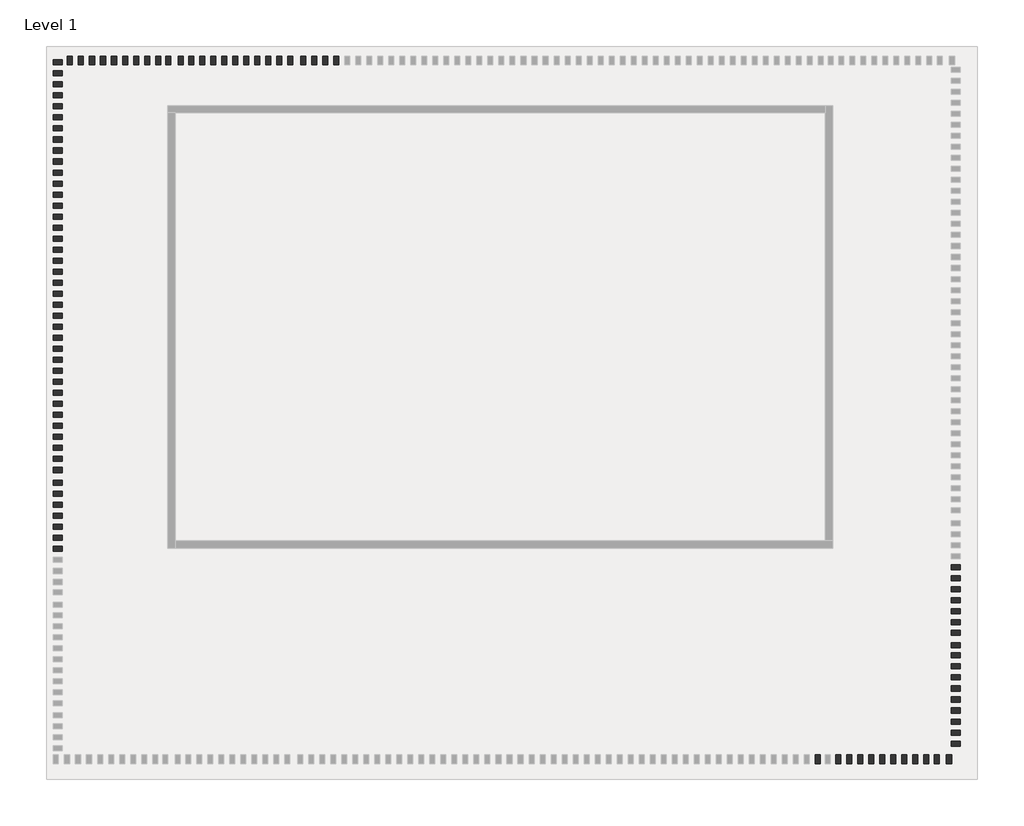
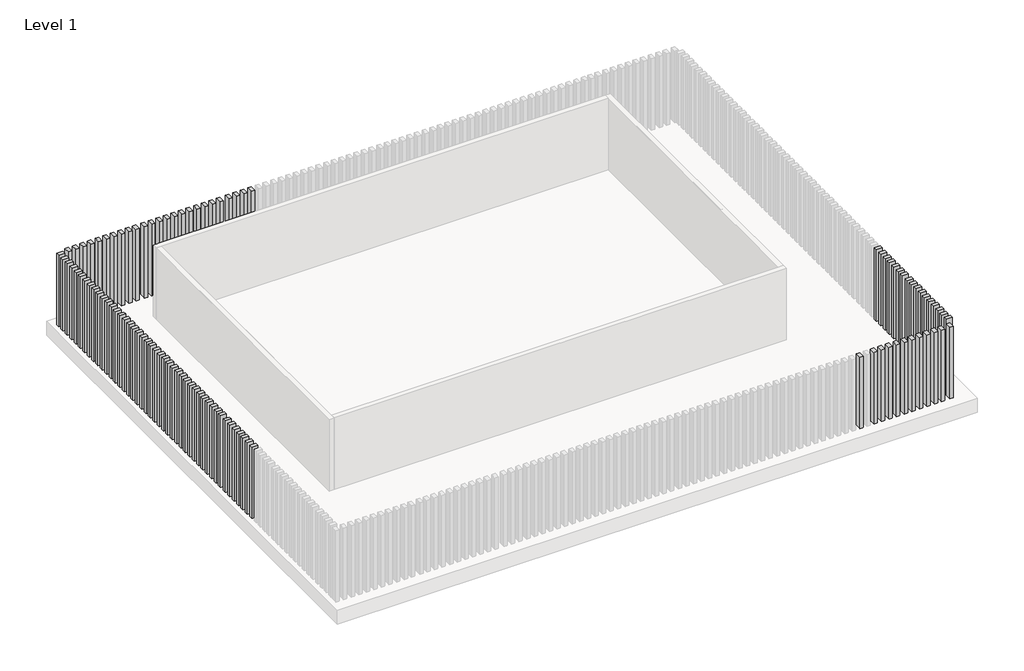
# One storey, part 2 of 3: 99 columns.
"""IFC4 building model written with IfcOpenShell, lengths in millimetres."""

from ifc_helpers import new_model, si_unit, origin, place, context, project, spatial, transform, mapped, element, save
from components import wood_timber_column_6_x_10_8585acab

model = new_model("IFC4")

# Units and contexts
model_context = context("Model", 3, world=origin())
ifc_project = project(units=[si_unit("LENGTHUNIT", "METRE", prefix="MILLI")], contexts=[model_context])

# Site, building, storey
site = spatial("IfcSite", under=ifc_project)
building = spatial("IfcBuilding", under=site)
storey = spatial("IfcBuildingStorey", under=building, Name="Level 1", Elevation=0.0)

# Columns
placement = place(None, origin())
wood_timber_column_6_x_10_shape = wood_timber_column_6_x_10_8585acab(model_context)
element("IfcColumn", 1, ObjectType="Wood Timber Column : 6 x 10", at=placement, inside=storey, context=model_context, shape_type="MappedRepresentation", body=[
    mapped(wood_timber_column_6_x_10_shape, transform((2270.6466756, -5612.3567338, 0.0), x_axis=(1.0, 0.0, 0.0), y_axis=(0.0, 1.0, 0.0), z_axis=(0.0, 0.0, 1.0))),
])
element("IfcColumn", 2, ObjectType="Wood Timber Column : 6 x 10", at=placement, inside=storey, context=model_context, shape_type="MappedRepresentation", body=[
    mapped(wood_timber_column_6_x_10_shape, transform((-18761.0148275, 13665.8652966, 0.0), x_axis=(0.0, 1.0, 0.0), y_axis=(-1.0000000000000002, 0.0, 0.0), z_axis=(0.0, 0.0, 1.0000000000000002))),
])
element("IfcColumn", 3, ObjectType="Wood Timber Column : 6 x 10", at=placement, inside=storey, context=model_context, shape_type="MappedRepresentation", body=[
    mapped(wood_timber_column_6_x_10_shape, transform((-18761.0148275, 13361.0652966, 0.0), x_axis=(0.0, 1.0, 0.0), y_axis=(-1.0000000000000002, 0.0, 0.0), z_axis=(0.0, 0.0, 1.0000000000000002))),
])
element("IfcColumn", 4, ObjectType="Wood Timber Column : 6 x 10", at=placement, inside=storey, context=model_context, shape_type="MappedRepresentation", body=[
    mapped(wood_timber_column_6_x_10_shape, transform((-18761.0148275, 13056.2652966, 0.0), x_axis=(0.0, 1.0, 0.0), y_axis=(-1.0000000000000002, 0.0, 0.0), z_axis=(0.0, 0.0, 1.0000000000000002))),
])
element("IfcColumn", 5, ObjectType="Wood Timber Column : 6 x 10", at=placement, inside=storey, context=model_context, shape_type="MappedRepresentation", body=[
    mapped(wood_timber_column_6_x_10_shape, transform((-18761.0148275, 12751.4652966, 0.0), x_axis=(0.0, 1.0, 0.0), y_axis=(-1.0000000000000002, 0.0, 0.0), z_axis=(0.0, 0.0, 1.0000000000000002))),
])
element("IfcColumn", 6, ObjectType="Wood Timber Column : 6 x 10", at=placement, inside=storey, context=model_context, shape_type="MappedRepresentation", body=[
    mapped(wood_timber_column_6_x_10_shape, transform((-18761.0148275, 12446.6652966, 0.0), x_axis=(0.0, 1.0, 0.0), y_axis=(-1.0000000000000002, 0.0, 0.0), z_axis=(0.0, 0.0, 1.0000000000000002))),
])
element("IfcColumn", 7, ObjectType="Wood Timber Column : 6 x 10", at=placement, inside=storey, context=model_context, shape_type="MappedRepresentation", body=[
    mapped(wood_timber_column_6_x_10_shape, transform((-18761.0148275, 12141.8652966, 0.0), x_axis=(0.0, 1.0, 0.0), y_axis=(-1.0000000000000002, 0.0, 0.0), z_axis=(0.0, 0.0, 1.0000000000000002))),
])
element("IfcColumn", 8, ObjectType="Wood Timber Column : 6 x 10", at=placement, inside=storey, context=model_context, shape_type="MappedRepresentation", body=[
    mapped(wood_timber_column_6_x_10_shape, transform((-18761.0148275, 11837.0652966, 0.0), x_axis=(0.0, 1.0, 0.0), y_axis=(-1.0000000000000002, 0.0, 0.0), z_axis=(0.0, 0.0, 1.0000000000000002))),
])
element("IfcColumn", 9, ObjectType="Wood Timber Column : 6 x 10", at=placement, inside=storey, context=model_context, shape_type="MappedRepresentation", body=[
    mapped(wood_timber_column_6_x_10_shape, transform((-18761.0148275, 11532.2652966, 0.0), x_axis=(0.0, 1.0, 0.0), y_axis=(-1.0000000000000002, 0.0, 0.0), z_axis=(0.0, 0.0, 1.0000000000000002))),
])
element("IfcColumn", 10, ObjectType="Wood Timber Column : 6 x 10", at=placement, inside=storey, context=model_context, shape_type="MappedRepresentation", body=[
    mapped(wood_timber_column_6_x_10_shape, transform((-18761.0148275, 11227.4652966, 0.0), x_axis=(0.0, 1.0, 0.0), y_axis=(-1.0000000000000002, 0.0, 0.0), z_axis=(0.0, 0.0, 1.0000000000000002))),
])
element("IfcColumn", 11, ObjectType="Wood Timber Column : 6 x 10", at=placement, inside=storey, context=model_context, shape_type="MappedRepresentation", body=[
    mapped(wood_timber_column_6_x_10_shape, transform((-18761.0148275, 10922.6652966, 0.0), x_axis=(0.0, 1.0, 0.0), y_axis=(-1.0000000000000002, 0.0, 0.0), z_axis=(0.0, 0.0, 1.0000000000000002))),
])
element("IfcColumn", 12, ObjectType="Wood Timber Column : 6 x 10", at=placement, inside=storey, context=model_context, shape_type="MappedRepresentation", body=[
    mapped(wood_timber_column_6_x_10_shape, transform((-18761.0148275, 10617.8652966, 0.0), x_axis=(0.0, 1.0, 0.0), y_axis=(-1.0000000000000002, 0.0, 0.0), z_axis=(0.0, 0.0, 1.0000000000000002))),
])
element("IfcColumn", 13, ObjectType="Wood Timber Column : 6 x 10", at=placement, inside=storey, context=model_context, shape_type="MappedRepresentation", body=[
    mapped(wood_timber_column_6_x_10_shape, transform((-18761.0148275, 10313.0652966, 0.0), x_axis=(0.0, 1.0, 0.0), y_axis=(-1.0000000000000002, 0.0, 0.0), z_axis=(0.0, 0.0, 1.0000000000000002))),
])
element("IfcColumn", 14, ObjectType="Wood Timber Column : 6 x 10", at=placement, inside=storey, context=model_context, shape_type="MappedRepresentation", body=[
    mapped(wood_timber_column_6_x_10_shape, transform((-18761.0148275, 10008.2652966, 0.0), x_axis=(0.0, 1.0, 0.0), y_axis=(-1.0000000000000002, 0.0, 0.0), z_axis=(0.0, 0.0, 1.0000000000000002))),
])
element("IfcColumn", 15, ObjectType="Wood Timber Column : 6 x 10", at=placement, inside=storey, context=model_context, shape_type="MappedRepresentation", body=[
    mapped(wood_timber_column_6_x_10_shape, transform((-18761.0148275, 9703.4652966, 0.0), x_axis=(0.0, 1.0, 0.0), y_axis=(-1.0000000000000002, 0.0, 0.0), z_axis=(0.0, 0.0, 1.0000000000000002))),
])
element("IfcColumn", 16, ObjectType="Wood Timber Column : 6 x 10", at=placement, inside=storey, context=model_context, shape_type="MappedRepresentation", body=[
    mapped(wood_timber_column_6_x_10_shape, transform((-18761.0148275, 9398.6652966, 0.0), x_axis=(0.0, 1.0, 0.0), y_axis=(-1.0000000000000002, 0.0, 0.0), z_axis=(0.0, 0.0, 1.0000000000000002))),
])
element("IfcColumn", 17, ObjectType="Wood Timber Column : 6 x 10", at=placement, inside=storey, context=model_context, shape_type="MappedRepresentation", body=[
    mapped(wood_timber_column_6_x_10_shape, transform((-18761.0148275, 9093.8652966, 0.0), x_axis=(0.0, 1.0, 0.0), y_axis=(-1.0000000000000002, 0.0, 0.0), z_axis=(0.0, 0.0, 1.0000000000000002))),
])
element("IfcColumn", 18, ObjectType="Wood Timber Column : 6 x 10", at=placement, inside=storey, context=model_context, shape_type="MappedRepresentation", body=[
    mapped(wood_timber_column_6_x_10_shape, transform((-18761.0148275, 8789.0652966, 0.0), x_axis=(0.0, 1.0, 0.0), y_axis=(-1.0000000000000002, 0.0, 0.0), z_axis=(0.0, 0.0, 1.0000000000000002))),
])
element("IfcColumn", 19, ObjectType="Wood Timber Column : 6 x 10", at=placement, inside=storey, context=model_context, shape_type="MappedRepresentation", body=[
    mapped(wood_timber_column_6_x_10_shape, transform((-18761.0148275, 8484.2652966, 0.0), x_axis=(0.0, 1.0, 0.0), y_axis=(-1.0000000000000002, 0.0, 0.0), z_axis=(0.0, 0.0, 1.0000000000000002))),
])
element("IfcColumn", 20, ObjectType="Wood Timber Column : 6 x 10", at=placement, inside=storey, context=model_context, shape_type="MappedRepresentation", body=[
    mapped(wood_timber_column_6_x_10_shape, transform((-18761.0148275, 8179.4652966, 0.0), x_axis=(0.0, 1.0, 0.0), y_axis=(-1.0000000000000002, 0.0, 0.0), z_axis=(0.0, 0.0, 1.0000000000000002))),
])
element("IfcColumn", 21, ObjectType="Wood Timber Column : 6 x 10", at=placement, inside=storey, context=model_context, shape_type="MappedRepresentation", body=[
    mapped(wood_timber_column_6_x_10_shape, transform((-18761.0148275, 7874.6652966, 0.0), x_axis=(0.0, 1.0, 0.0), y_axis=(-1.0000000000000002, 0.0, 0.0), z_axis=(0.0, 0.0, 1.0000000000000002))),
])
element("IfcColumn", 22, ObjectType="Wood Timber Column : 6 x 10", at=placement, inside=storey, context=model_context, shape_type="MappedRepresentation", body=[
    mapped(wood_timber_column_6_x_10_shape, transform((-18761.0148275, 7569.8652966, 0.0), x_axis=(0.0, 1.0, 0.0), y_axis=(-1.0000000000000002, 0.0, 0.0), z_axis=(0.0, 0.0, 1.0000000000000002))),
])
element("IfcColumn", 23, ObjectType="Wood Timber Column : 6 x 10", at=placement, inside=storey, context=model_context, shape_type="MappedRepresentation", body=[
    mapped(wood_timber_column_6_x_10_shape, transform((-18761.0148275, 7265.0652966, 0.0), x_axis=(0.0, 1.0, 0.0), y_axis=(-1.0000000000000002, 0.0, 0.0), z_axis=(0.0, 0.0, 1.0000000000000002))),
])
element("IfcColumn", 24, ObjectType="Wood Timber Column : 6 x 10", at=placement, inside=storey, context=model_context, shape_type="MappedRepresentation", body=[
    mapped(wood_timber_column_6_x_10_shape, transform((-18761.0148275, 6960.2652966, 0.0), x_axis=(0.0, 1.0, 0.0), y_axis=(-1.0000000000000002, 0.0, 0.0), z_axis=(0.0, 0.0, 1.0000000000000002))),
])
element("IfcColumn", 25, ObjectType="Wood Timber Column : 6 x 10", at=placement, inside=storey, context=model_context, shape_type="MappedRepresentation", body=[
    mapped(wood_timber_column_6_x_10_shape, transform((-18761.0148275, 6655.4652966, 0.0), x_axis=(0.0, 1.0, 0.0), y_axis=(-1.0000000000000002, 0.0, 0.0), z_axis=(0.0, 0.0, 1.0000000000000002))),
])
element("IfcColumn", 26, ObjectType="Wood Timber Column : 6 x 10", at=placement, inside=storey, context=model_context, shape_type="MappedRepresentation", body=[
    mapped(wood_timber_column_6_x_10_shape, transform((-18761.0148275, 6350.6652966, 0.0), x_axis=(0.0, 1.0, 0.0), y_axis=(-1.0000000000000002, 0.0, 0.0), z_axis=(0.0, 0.0, 1.0000000000000002))),
])
element("IfcColumn", 27, ObjectType="Wood Timber Column : 6 x 10", at=placement, inside=storey, context=model_context, shape_type="MappedRepresentation", body=[
    mapped(wood_timber_column_6_x_10_shape, transform((-18761.0148275, 6045.8652966, 0.0), x_axis=(0.0, 1.0, 0.0), y_axis=(-1.0000000000000002, 0.0, 0.0), z_axis=(0.0, 0.0, 1.0000000000000002))),
])
element("IfcColumn", 28, ObjectType="Wood Timber Column : 6 x 10", at=placement, inside=storey, context=model_context, shape_type="MappedRepresentation", body=[
    mapped(wood_timber_column_6_x_10_shape, transform((-18761.0148275, 5741.0652966, 0.0), x_axis=(0.0, 1.0, 0.0), y_axis=(-1.0000000000000002, 0.0, 0.0), z_axis=(0.0, 0.0, 1.0000000000000002))),
])
element("IfcColumn", 29, ObjectType="Wood Timber Column : 6 x 10", at=placement, inside=storey, context=model_context, shape_type="MappedRepresentation", body=[
    mapped(wood_timber_column_6_x_10_shape, transform((-18761.0148275, 5436.2652966, 0.0), x_axis=(0.0, 1.0, 0.0), y_axis=(-1.0000000000000002, 0.0, 0.0), z_axis=(0.0, 0.0, 1.0000000000000002))),
])
element("IfcColumn", 30, ObjectType="Wood Timber Column : 6 x 10", at=placement, inside=storey, context=model_context, shape_type="MappedRepresentation", body=[
    mapped(wood_timber_column_6_x_10_shape, transform((-18761.0148275, 5131.4652966, 0.0), x_axis=(0.0, 1.0, 0.0), y_axis=(-1.0000000000000002, 0.0, 0.0), z_axis=(0.0, 0.0, 1.0000000000000002))),
])
element("IfcColumn", 31, ObjectType="Wood Timber Column : 6 x 10", at=placement, inside=storey, context=model_context, shape_type="MappedRepresentation", body=[
    mapped(wood_timber_column_6_x_10_shape, transform((-18761.0148275, 4826.6652966, 0.0), x_axis=(0.0, 1.0, 0.0), y_axis=(-1.0000000000000002, 0.0, 0.0), z_axis=(0.0, 0.0, 1.0000000000000002))),
])
element("IfcColumn", 32, ObjectType="Wood Timber Column : 6 x 10", at=placement, inside=storey, context=model_context, shape_type="MappedRepresentation", body=[
    mapped(wood_timber_column_6_x_10_shape, transform((-18761.0148275, 4521.8652966, 0.0), x_axis=(0.0, 1.0, 0.0), y_axis=(-1.0000000000000002, 0.0, 0.0), z_axis=(0.0, 0.0, 1.0000000000000002))),
])
element("IfcColumn", 33, ObjectType="Wood Timber Column : 6 x 10", at=placement, inside=storey, context=model_context, shape_type="MappedRepresentation", body=[
    mapped(wood_timber_column_6_x_10_shape, transform((-18761.0148275, 4217.0652966, 0.0), x_axis=(0.0, 1.0, 0.0), y_axis=(-1.0000000000000002, 0.0, 0.0), z_axis=(0.0, 0.0, 1.0000000000000002))),
])
element("IfcColumn", 34, ObjectType="Wood Timber Column : 6 x 10", at=placement, inside=storey, context=model_context, shape_type="MappedRepresentation", body=[
    mapped(wood_timber_column_6_x_10_shape, transform((-18761.0148275, 3912.2652966, 0.0), x_axis=(0.0, 1.0, 0.0), y_axis=(-1.0000000000000002, 0.0, 0.0), z_axis=(0.0, 0.0, 1.0000000000000002))),
])
element("IfcColumn", 35, ObjectType="Wood Timber Column : 6 x 10", at=placement, inside=storey, context=model_context, shape_type="MappedRepresentation", body=[
    mapped(wood_timber_column_6_x_10_shape, transform((-18761.0148275, 3607.4652966, 0.0), x_axis=(0.0, 1.0, 0.0), y_axis=(-1.0000000000000002, 0.0, 0.0), z_axis=(0.0, 0.0, 1.0000000000000002))),
])
element("IfcColumn", 36, ObjectType="Wood Timber Column : 6 x 10", at=placement, inside=storey, context=model_context, shape_type="MappedRepresentation", body=[
    mapped(wood_timber_column_6_x_10_shape, transform((-18761.0148275, 3302.6652966, 0.0), x_axis=(0.0, 1.0, 0.0), y_axis=(-1.0000000000000002, 0.0, 0.0), z_axis=(0.0, 0.0, 1.0000000000000002))),
])
element("IfcColumn", 37, ObjectType="Wood Timber Column : 6 x 10", at=placement, inside=storey, context=model_context, shape_type="MappedRepresentation", body=[
    mapped(wood_timber_column_6_x_10_shape, transform((-18761.0148275, 2997.8652966, 0.0), x_axis=(0.0, 1.0, 0.0), y_axis=(-1.0000000000000002, 0.0, 0.0), z_axis=(0.0, 0.0, 1.0000000000000002))),
])
element("IfcColumn", 38, ObjectType="Wood Timber Column : 6 x 10", at=placement, inside=storey, context=model_context, shape_type="MappedRepresentation", body=[
    mapped(wood_timber_column_6_x_10_shape, transform((-18761.0148275, 2693.0652966, 0.0), x_axis=(0.0, 1.0, 0.0), y_axis=(-1.0000000000000002, 0.0, 0.0), z_axis=(0.0, 0.0, 1.0000000000000002))),
])
element("IfcColumn", 39, ObjectType="Wood Timber Column : 6 x 10", at=placement, inside=storey, context=model_context, shape_type="MappedRepresentation", body=[
    mapped(wood_timber_column_6_x_10_shape, transform((-18761.0148275, 2388.2652966, 0.0), x_axis=(0.0, 1.0, 0.0), y_axis=(-1.0000000000000002, 0.0, 0.0), z_axis=(0.0, 0.0, 1.0000000000000002))),
])
element("IfcColumn", 40, ObjectType="Wood Timber Column : 6 x 10", at=placement, inside=storey, context=model_context, shape_type="MappedRepresentation", body=[
    mapped(wood_timber_column_6_x_10_shape, transform((-18761.0148275, 2032.6652966, 0.0), x_axis=(0.0, 1.0, 0.0), y_axis=(-1.0000000000000002, 0.0, 0.0), z_axis=(0.0, 0.0, 1.0000000000000002))),
])
element("IfcColumn", 41, ObjectType="Wood Timber Column : 6 x 10", at=placement, inside=storey, context=model_context, shape_type="MappedRepresentation", body=[
    mapped(wood_timber_column_6_x_10_shape, transform((-18761.0148275, 1727.8652966, 0.0), x_axis=(0.0, 1.0, 0.0), y_axis=(-1.0000000000000002, 0.0, 0.0), z_axis=(0.0, 0.0, 1.0000000000000002))),
])
element("IfcColumn", 42, ObjectType="Wood Timber Column : 6 x 10", at=placement, inside=storey, context=model_context, shape_type="MappedRepresentation", body=[
    mapped(wood_timber_column_6_x_10_shape, transform((-18761.0148275, 1423.0652966, 0.0), x_axis=(0.0, 1.0, 0.0), y_axis=(-1.0000000000000002, 0.0, 0.0), z_axis=(0.0, 0.0, 1.0000000000000002))),
])
element("IfcColumn", 43, ObjectType="Wood Timber Column : 6 x 10", at=placement, inside=storey, context=model_context, shape_type="MappedRepresentation", body=[
    mapped(wood_timber_column_6_x_10_shape, transform((-18761.0148275, 1118.2652966, 0.0), x_axis=(0.0, 1.0, 0.0), y_axis=(-1.0000000000000002, 0.0, 0.0), z_axis=(0.0, 0.0, 1.0000000000000002))),
])
element("IfcColumn", 44, ObjectType="Wood Timber Column : 6 x 10", at=placement, inside=storey, context=model_context, shape_type="MappedRepresentation", body=[
    mapped(wood_timber_column_6_x_10_shape, transform((-18761.0148275, 813.4652966, 0.0), x_axis=(0.0, 1.0, 0.0), y_axis=(-1.0000000000000002, 0.0, 0.0), z_axis=(0.0, 0.0, 1.0000000000000002))),
])
element("IfcColumn", 45, ObjectType="Wood Timber Column : 6 x 10", at=placement, inside=storey, context=model_context, shape_type="MappedRepresentation", body=[
    mapped(wood_timber_column_6_x_10_shape, transform((-18761.0148275, 508.6652966, 0.0), x_axis=(0.0, 1.0, 0.0), y_axis=(-1.0000000000000002, 0.0, 0.0), z_axis=(0.0, 0.0, 1.0000000000000002))),
])
element("IfcColumn", 46, ObjectType="Wood Timber Column : 6 x 10", at=placement, inside=storey, context=model_context, shape_type="MappedRepresentation", body=[
    mapped(wood_timber_column_6_x_10_shape, transform((-18761.0148275, 203.8652966, 0.0), x_axis=(0.0, 1.0, 0.0), y_axis=(-1.0000000000000002, 0.0, 0.0), z_axis=(0.0, 0.0, 1.0000000000000002))),
])
element("IfcColumn", 47, ObjectType="Wood Timber Column : 6 x 10", at=placement, inside=storey, context=model_context, shape_type="MappedRepresentation", body=[
    mapped(wood_timber_column_6_x_10_shape, transform((6080.1851725, -304.1347034, 0.0), x_axis=(0.0, 1.0, 0.0), y_axis=(-1.0000000000000002, 0.0, 0.0), z_axis=(0.0, 0.0, 1.0000000000000002))),
])
element("IfcColumn", 48, ObjectType="Wood Timber Column : 6 x 10", at=placement, inside=storey, context=model_context, shape_type="MappedRepresentation", body=[
    mapped(wood_timber_column_6_x_10_shape, transform((6080.1851725, -608.9347034, 0.0), x_axis=(0.0, 1.0, 0.0), y_axis=(-1.0000000000000002, 0.0, 0.0), z_axis=(0.0, 0.0, 1.0000000000000002))),
])
element("IfcColumn", 49, ObjectType="Wood Timber Column : 6 x 10", at=placement, inside=storey, context=model_context, shape_type="MappedRepresentation", body=[
    mapped(wood_timber_column_6_x_10_shape, transform((6080.1851725, -913.7347034, 0.0), x_axis=(0.0, 1.0, 0.0), y_axis=(-1.0000000000000002, 0.0, 0.0), z_axis=(0.0, 0.0, 1.0000000000000002))),
])
element("IfcColumn", 50, ObjectType="Wood Timber Column : 6 x 10", at=placement, inside=storey, context=model_context, shape_type="MappedRepresentation", body=[
    mapped(wood_timber_column_6_x_10_shape, transform((6080.1851725, -1218.5347034, 0.0), x_axis=(0.0, 1.0, 0.0), y_axis=(-1.0000000000000002, 0.0, 0.0), z_axis=(0.0, 0.0, 1.0000000000000002))),
])
element("IfcColumn", 51, ObjectType="Wood Timber Column : 6 x 10", at=placement, inside=storey, context=model_context, shape_type="MappedRepresentation", body=[
    mapped(wood_timber_column_6_x_10_shape, transform((6080.1851725, -1523.3347034, 0.0), x_axis=(0.0, 1.0, 0.0), y_axis=(-1.0000000000000002, 0.0, 0.0), z_axis=(0.0, 0.0, 1.0000000000000002))),
])
element("IfcColumn", 52, ObjectType="Wood Timber Column : 6 x 10", at=placement, inside=storey, context=model_context, shape_type="MappedRepresentation", body=[
    mapped(wood_timber_column_6_x_10_shape, transform((6080.1851725, -1828.1347034, 0.0), x_axis=(0.0, 1.0, 0.0), y_axis=(-1.0000000000000002, 0.0, 0.0), z_axis=(0.0, 0.0, 1.0000000000000002))),
])
element("IfcColumn", 53, ObjectType="Wood Timber Column : 6 x 10", at=placement, inside=storey, context=model_context, shape_type="MappedRepresentation", body=[
    mapped(wood_timber_column_6_x_10_shape, transform((6080.1851725, -2113.8847034, 0.0), x_axis=(0.0, 1.0, 0.0), y_axis=(-1.0000000000000002, 0.0, 0.0), z_axis=(0.0, 0.0, 1.0000000000000002))),
])
element("IfcColumn", 54, ObjectType="Wood Timber Column : 6 x 10", at=placement, inside=storey, context=model_context, shape_type="MappedRepresentation", body=[
    mapped(wood_timber_column_6_x_10_shape, transform((6080.1851725, -2456.7847034, 0.0), x_axis=(0.0, 1.0, 0.0), y_axis=(-1.0000000000000002, 0.0, 0.0), z_axis=(0.0, 0.0, 1.0000000000000002))),
])
element("IfcColumn", 55, ObjectType="Wood Timber Column : 6 x 10", at=placement, inside=storey, context=model_context, shape_type="MappedRepresentation", body=[
    mapped(wood_timber_column_6_x_10_shape, transform((6080.1851725, -2742.5347034, 0.0), x_axis=(0.0, 1.0, 0.0), y_axis=(-1.0000000000000002, 0.0, 0.0), z_axis=(0.0, 0.0, 1.0000000000000002))),
])
element("IfcColumn", 56, ObjectType="Wood Timber Column : 6 x 10", at=placement, inside=storey, context=model_context, shape_type="MappedRepresentation", body=[
    mapped(wood_timber_column_6_x_10_shape, transform((6080.1851725, -3047.3347034, 0.0), x_axis=(0.0, 1.0, 0.0), y_axis=(-1.0000000000000002, 0.0, 0.0), z_axis=(0.0, 0.0, 1.0000000000000002))),
])
element("IfcColumn", 57, ObjectType="Wood Timber Column : 6 x 10", at=placement, inside=storey, context=model_context, shape_type="MappedRepresentation", body=[
    mapped(wood_timber_column_6_x_10_shape, transform((6080.1851725, -3352.1347034, 0.0), x_axis=(0.0, 1.0, 0.0), y_axis=(-1.0000000000000002, 0.0, 0.0), z_axis=(0.0, 0.0, 1.0000000000000002))),
])
element("IfcColumn", 58, ObjectType="Wood Timber Column : 6 x 10", at=placement, inside=storey, context=model_context, shape_type="MappedRepresentation", body=[
    mapped(wood_timber_column_6_x_10_shape, transform((6080.1851725, -3656.9347034, 0.0), x_axis=(0.0, 1.0, 0.0), y_axis=(-1.0000000000000002, 0.0, 0.0), z_axis=(0.0, 0.0, 1.0000000000000002))),
])
element("IfcColumn", 59, ObjectType="Wood Timber Column : 6 x 10", at=placement, inside=storey, context=model_context, shape_type="MappedRepresentation", body=[
    mapped(wood_timber_column_6_x_10_shape, transform((6080.1851725, -3961.7347034, 0.0), x_axis=(0.0, 1.0, 0.0), y_axis=(-1.0000000000000002, 0.0, 0.0), z_axis=(0.0, 0.0, 1.0000000000000002))),
])
element("IfcColumn", 60, ObjectType="Wood Timber Column : 6 x 10", at=placement, inside=storey, context=model_context, shape_type="MappedRepresentation", body=[
    mapped(wood_timber_column_6_x_10_shape, transform((6080.1851725, -4266.5347034, 0.0), x_axis=(0.0, 1.0, 0.0), y_axis=(-1.0000000000000002, 0.0, 0.0), z_axis=(0.0, 0.0, 1.0000000000000002))),
])
element("IfcColumn", 61, ObjectType="Wood Timber Column : 6 x 10", at=placement, inside=storey, context=model_context, shape_type="MappedRepresentation", body=[
    mapped(wood_timber_column_6_x_10_shape, transform((6080.1851725, -4571.3347034, 0.0), x_axis=(0.0, 1.0, 0.0), y_axis=(-1.0000000000000002, 0.0, 0.0), z_axis=(0.0, 0.0, 1.0000000000000002))),
])
element("IfcColumn", 62, ObjectType="Wood Timber Column : 6 x 10", at=placement, inside=storey, context=model_context, shape_type="MappedRepresentation", body=[
    mapped(wood_timber_column_6_x_10_shape, transform((6080.1851725, -4876.1347034, 0.0), x_axis=(0.0, 1.0, 0.0), y_axis=(-1.0000000000000002, 0.0, 0.0), z_axis=(0.0, 0.0, 1.0000000000000002))),
])
element("IfcColumn", 63, ObjectType="Wood Timber Column : 6 x 10", at=placement, inside=storey, context=model_context, shape_type="MappedRepresentation", body=[
    mapped(wood_timber_column_6_x_10_shape, transform((6080.1851725, -5180.9347034, 0.0), x_axis=(0.0, 1.0, 0.0), y_axis=(-1.0000000000000002, 0.0, 0.0), z_axis=(0.0, 0.0, 1.0000000000000002))),
])
element("IfcColumn", 64, ObjectType="Wood Timber Column : 6 x 10", at=placement, inside=storey, context=model_context, shape_type="MappedRepresentation", body=[
    mapped(wood_timber_column_6_x_10_shape, transform((5896.4966756, -5612.3567338, 0.0), x_axis=(1.0, 0.0, 0.0), y_axis=(0.0, 1.0, 0.0), z_axis=(0.0, 0.0, 1.0))),
])
element("IfcColumn", 65, ObjectType="Wood Timber Column : 6 x 10", at=placement, inside=storey, context=model_context, shape_type="MappedRepresentation", body=[
    mapped(wood_timber_column_6_x_10_shape, transform((5553.5966756, -5612.3567338, 0.0), x_axis=(1.0, 0.0, 0.0), y_axis=(0.0, 1.0, 0.0), z_axis=(0.0, 0.0, 1.0))),
])
element("IfcColumn", 66, ObjectType="Wood Timber Column : 6 x 10", at=placement, inside=storey, context=model_context, shape_type="MappedRepresentation", body=[
    mapped(wood_timber_column_6_x_10_shape, transform((5267.8466756, -5612.3567338, 0.0), x_axis=(1.0, 0.0, 0.0), y_axis=(0.0, 1.0, 0.0), z_axis=(0.0, 0.0, 1.0))),
])
element("IfcColumn", 67, ObjectType="Wood Timber Column : 6 x 10", at=placement, inside=storey, context=model_context, shape_type="MappedRepresentation", body=[
    mapped(wood_timber_column_6_x_10_shape, transform((4963.0466756, -5612.3567338, 0.0), x_axis=(1.0, 0.0, 0.0), y_axis=(0.0, 1.0, 0.0), z_axis=(0.0, 0.0, 1.0))),
])
element("IfcColumn", 68, ObjectType="Wood Timber Column : 6 x 10", at=placement, inside=storey, context=model_context, shape_type="MappedRepresentation", body=[
    mapped(wood_timber_column_6_x_10_shape, transform((4658.2466756, -5612.3567338, 0.0), x_axis=(1.0, 0.0, 0.0), y_axis=(0.0, 1.0, 0.0), z_axis=(0.0, 0.0, 1.0))),
])
element("IfcColumn", 69, ObjectType="Wood Timber Column : 6 x 10", at=placement, inside=storey, context=model_context, shape_type="MappedRepresentation", body=[
    mapped(wood_timber_column_6_x_10_shape, transform((4353.4466756, -5612.3567338, 0.0), x_axis=(1.0, 0.0, 0.0), y_axis=(0.0, 1.0, 0.0), z_axis=(0.0, 0.0, 1.0))),
])
element("IfcColumn", 70, ObjectType="Wood Timber Column : 6 x 10", at=placement, inside=storey, context=model_context, shape_type="MappedRepresentation", body=[
    mapped(wood_timber_column_6_x_10_shape, transform((4048.6466756, -5612.3567338, 0.0), x_axis=(1.0, 0.0, 0.0), y_axis=(0.0, 1.0, 0.0), z_axis=(0.0, 0.0, 1.0))),
])
element("IfcColumn", 71, ObjectType="Wood Timber Column : 6 x 10", at=placement, inside=storey, context=model_context, shape_type="MappedRepresentation", body=[
    mapped(wood_timber_column_6_x_10_shape, transform((3743.8466756, -5612.3567338, 0.0), x_axis=(1.0, 0.0, 0.0), y_axis=(0.0, 1.0, 0.0), z_axis=(0.0, 0.0, 1.0))),
])
element("IfcColumn", 72, ObjectType="Wood Timber Column : 6 x 10", at=placement, inside=storey, context=model_context, shape_type="MappedRepresentation", body=[
    mapped(wood_timber_column_6_x_10_shape, transform((3439.0466756, -5612.3567338, 0.0), x_axis=(1.0, 0.0, 0.0), y_axis=(0.0, 1.0, 0.0), z_axis=(0.0, 0.0, 1.0))),
])
element("IfcColumn", 73, ObjectType="Wood Timber Column : 6 x 10", at=placement, inside=storey, context=model_context, shape_type="MappedRepresentation", body=[
    mapped(wood_timber_column_6_x_10_shape, transform((3134.2466756, -5612.3567338, 0.0), x_axis=(1.0, 0.0, 0.0), y_axis=(0.0, 1.0, 0.0), z_axis=(0.0, 0.0, 1.0))),
])
element("IfcColumn", 74, ObjectType="Wood Timber Column : 6 x 10", at=placement, inside=storey, context=model_context, shape_type="MappedRepresentation", body=[
    mapped(wood_timber_column_6_x_10_shape, transform((2829.4466756, -5612.3567338, 0.0), x_axis=(1.0, 0.0, 0.0), y_axis=(0.0, 1.0, 0.0), z_axis=(0.0, 0.0, 1.0))),
])
element("IfcColumn", 75, ObjectType="Wood Timber Column : 6 x 10", at=placement, inside=storey, context=model_context, shape_type="MappedRepresentation", body=[
    mapped(wood_timber_column_6_x_10_shape, transform((-11058.4648275, 13716.6652966, 0.0), x_axis=(1.0, 0.0, 0.0), y_axis=(0.0, 1.0, 0.0), z_axis=(0.0, 0.0, 1.0))),
])
element("IfcColumn", 76, ObjectType="Wood Timber Column : 6 x 10", at=placement, inside=storey, context=model_context, shape_type="MappedRepresentation", body=[
    mapped(wood_timber_column_6_x_10_shape, transform((-11363.2648275, 13716.6652966, 0.0), x_axis=(1.0, 0.0, 0.0), y_axis=(0.0, 1.0, 0.0), z_axis=(0.0, 0.0, 1.0))),
])
element("IfcColumn", 77, ObjectType="Wood Timber Column : 6 x 10", at=placement, inside=storey, context=model_context, shape_type="MappedRepresentation", body=[
    mapped(wood_timber_column_6_x_10_shape, transform((-11668.0648275, 13716.6652966, 0.0), x_axis=(1.0, 0.0, 0.0), y_axis=(0.0, 1.0, 0.0), z_axis=(0.0, 0.0, 1.0))),
])
element("IfcColumn", 78, ObjectType="Wood Timber Column : 6 x 10", at=placement, inside=storey, context=model_context, shape_type="MappedRepresentation", body=[
    mapped(wood_timber_column_6_x_10_shape, transform((-11972.8648275, 13716.6652966, 0.0), x_axis=(1.0, 0.0, 0.0), y_axis=(0.0, 1.0, 0.0), z_axis=(0.0, 0.0, 1.0))),
])
element("IfcColumn", 79, ObjectType="Wood Timber Column : 6 x 10", at=placement, inside=storey, context=model_context, shape_type="MappedRepresentation", body=[
    mapped(wood_timber_column_6_x_10_shape, transform((-12328.4648275, 13716.6652966, 0.0), x_axis=(1.0, 0.0, 0.0), y_axis=(0.0, 1.0, 0.0), z_axis=(0.0, 0.0, 1.0))),
])
element("IfcColumn", 80, ObjectType="Wood Timber Column : 6 x 10", at=placement, inside=storey, context=model_context, shape_type="MappedRepresentation", body=[
    mapped(wood_timber_column_6_x_10_shape, transform((-12633.2648275, 13716.6652966, 0.0), x_axis=(1.0, 0.0, 0.0), y_axis=(0.0, 1.0, 0.0), z_axis=(0.0, 0.0, 1.0))),
])
element("IfcColumn", 81, ObjectType="Wood Timber Column : 6 x 10", at=placement, inside=storey, context=model_context, shape_type="MappedRepresentation", body=[
    mapped(wood_timber_column_6_x_10_shape, transform((-12938.0648275, 13716.6652966, 0.0), x_axis=(1.0, 0.0, 0.0), y_axis=(0.0, 1.0, 0.0), z_axis=(0.0, 0.0, 1.0))),
])
element("IfcColumn", 82, ObjectType="Wood Timber Column : 6 x 10", at=placement, inside=storey, context=model_context, shape_type="MappedRepresentation", body=[
    mapped(wood_timber_column_6_x_10_shape, transform((-13242.8648275, 13716.6652966, 0.0), x_axis=(1.0, 0.0, 0.0), y_axis=(0.0, 1.0, 0.0), z_axis=(0.0, 0.0, 1.0))),
])
element("IfcColumn", 83, ObjectType="Wood Timber Column : 6 x 10", at=placement, inside=storey, context=model_context, shape_type="MappedRepresentation", body=[
    mapped(wood_timber_column_6_x_10_shape, transform((-13547.6648275, 13716.6652966, 0.0), x_axis=(1.0, 0.0, 0.0), y_axis=(0.0, 1.0, 0.0), z_axis=(0.0, 0.0, 1.0))),
])
element("IfcColumn", 84, ObjectType="Wood Timber Column : 6 x 10", at=placement, inside=storey, context=model_context, shape_type="MappedRepresentation", body=[
    mapped(wood_timber_column_6_x_10_shape, transform((-13852.4648275, 13716.6652966, 0.0), x_axis=(1.0, 0.0, 0.0), y_axis=(0.0, 1.0, 0.0), z_axis=(0.0, 0.0, 1.0))),
])
element("IfcColumn", 85, ObjectType="Wood Timber Column : 6 x 10", at=placement, inside=storey, context=model_context, shape_type="MappedRepresentation", body=[
    mapped(wood_timber_column_6_x_10_shape, transform((-14157.2648275, 13716.6652966, 0.0), x_axis=(1.0, 0.0, 0.0), y_axis=(0.0, 1.0, 0.0), z_axis=(0.0, 0.0, 1.0))),
])
element("IfcColumn", 86, ObjectType="Wood Timber Column : 6 x 10", at=placement, inside=storey, context=model_context, shape_type="MappedRepresentation", body=[
    mapped(wood_timber_column_6_x_10_shape, transform((-14462.0648275, 13716.6652966, 0.0), x_axis=(1.0, 0.0, 0.0), y_axis=(0.0, 1.0, 0.0), z_axis=(0.0, 0.0, 1.0))),
])
element("IfcColumn", 87, ObjectType="Wood Timber Column : 6 x 10", at=placement, inside=storey, context=model_context, shape_type="MappedRepresentation", body=[
    mapped(wood_timber_column_6_x_10_shape, transform((-14766.8648275, 13716.6652966, 0.0), x_axis=(1.0, 0.0, 0.0), y_axis=(0.0, 1.0, 0.0), z_axis=(0.0, 0.0, 1.0))),
])
element("IfcColumn", 88, ObjectType="Wood Timber Column : 6 x 10", at=placement, inside=storey, context=model_context, shape_type="MappedRepresentation", body=[
    mapped(wood_timber_column_6_x_10_shape, transform((-15071.6648275, 13716.6652966, 0.0), x_axis=(1.0, 0.0, 0.0), y_axis=(0.0, 1.0, 0.0), z_axis=(0.0, 0.0, 1.0))),
])
element("IfcColumn", 89, ObjectType="Wood Timber Column : 6 x 10", at=placement, inside=storey, context=model_context, shape_type="MappedRepresentation", body=[
    mapped(wood_timber_column_6_x_10_shape, transform((-15357.4148275, 13716.6652966, 0.0), x_axis=(1.0, 0.0, 0.0), y_axis=(0.0, 1.0, 0.0), z_axis=(0.0, 0.0, 1.0))),
])
element("IfcColumn", 90, ObjectType="Wood Timber Column : 6 x 10", at=placement, inside=storey, context=model_context, shape_type="MappedRepresentation", body=[
    mapped(wood_timber_column_6_x_10_shape, transform((-15700.3148275, 13716.6652966, 0.0), x_axis=(1.0, 0.0, 0.0), y_axis=(0.0, 1.0, 0.0), z_axis=(0.0, 0.0, 1.0))),
])
element("IfcColumn", 91, ObjectType="Wood Timber Column : 6 x 10", at=placement, inside=storey, context=model_context, shape_type="MappedRepresentation", body=[
    mapped(wood_timber_column_6_x_10_shape, transform((-15986.0648275, 13716.6652966, 0.0), x_axis=(1.0, 0.0, 0.0), y_axis=(0.0, 1.0, 0.0), z_axis=(0.0, 0.0, 1.0))),
])
element("IfcColumn", 92, ObjectType="Wood Timber Column : 6 x 10", at=placement, inside=storey, context=model_context, shape_type="MappedRepresentation", body=[
    mapped(wood_timber_column_6_x_10_shape, transform((-16290.8648275, 13716.6652966, 0.0), x_axis=(1.0, 0.0, 0.0), y_axis=(0.0, 1.0, 0.0), z_axis=(0.0, 0.0, 1.0))),
])
element("IfcColumn", 93, ObjectType="Wood Timber Column : 6 x 10", at=placement, inside=storey, context=model_context, shape_type="MappedRepresentation", body=[
    mapped(wood_timber_column_6_x_10_shape, transform((-16595.6648275, 13716.6652966, 0.0), x_axis=(1.0, 0.0, 0.0), y_axis=(0.0, 1.0, 0.0), z_axis=(0.0, 0.0, 1.0))),
])
element("IfcColumn", 94, ObjectType="Wood Timber Column : 6 x 10", at=placement, inside=storey, context=model_context, shape_type="MappedRepresentation", body=[
    mapped(wood_timber_column_6_x_10_shape, transform((-16900.4648275, 13716.6652966, 0.0), x_axis=(1.0, 0.0, 0.0), y_axis=(0.0, 1.0, 0.0), z_axis=(0.0, 0.0, 1.0))),
])
element("IfcColumn", 95, ObjectType="Wood Timber Column : 6 x 10", at=placement, inside=storey, context=model_context, shape_type="MappedRepresentation", body=[
    mapped(wood_timber_column_6_x_10_shape, transform((-17205.2648275, 13716.6652966, 0.0), x_axis=(1.0, 0.0, 0.0), y_axis=(0.0, 1.0, 0.0), z_axis=(0.0, 0.0, 1.0))),
])
element("IfcColumn", 96, ObjectType="Wood Timber Column : 6 x 10", at=placement, inside=storey, context=model_context, shape_type="MappedRepresentation", body=[
    mapped(wood_timber_column_6_x_10_shape, transform((-17510.0648275, 13716.6652966, 0.0), x_axis=(1.0, 0.0, 0.0), y_axis=(0.0, 1.0, 0.0), z_axis=(0.0, 0.0, 1.0))),
])
element("IfcColumn", 97, ObjectType="Wood Timber Column : 6 x 10", at=placement, inside=storey, context=model_context, shape_type="MappedRepresentation", body=[
    mapped(wood_timber_column_6_x_10_shape, transform((-17814.8648275, 13716.6652966, 0.0), x_axis=(1.0, 0.0, 0.0), y_axis=(0.0, 1.0, 0.0), z_axis=(0.0, 0.0, 1.0))),
])
element("IfcColumn", 98, ObjectType="Wood Timber Column : 6 x 10", at=placement, inside=storey, context=model_context, shape_type="MappedRepresentation", body=[
    mapped(wood_timber_column_6_x_10_shape, transform((-18119.6648275, 13716.6652966, 0.0), x_axis=(1.0, 0.0, 0.0), y_axis=(0.0, 1.0, 0.0), z_axis=(0.0, 0.0, 1.0))),
])
element("IfcColumn", 99, ObjectType="Wood Timber Column : 6 x 10", at=placement, inside=storey, context=model_context, shape_type="MappedRepresentation", body=[
    mapped(wood_timber_column_6_x_10_shape, transform((-18424.4648275, 13716.6652966, 0.0), x_axis=(1.0, 0.0, 0.0), y_axis=(0.0, 1.0, 0.0), z_axis=(0.0, 0.0, 1.0))),
])

save(model, "model.ifc")

# Revit data of these elements
# Type "Wood Timber Column : 6 x 10"
#   Assembly Code = "B1010200"
#   Depth = 0' - 9 1/2"
#   Width = 0' - 5 1/2"
#   Material = Softwood, Lumber
# Elements 1, 2, 3, 4, 5, 6, 7, 8, 9, 10, 11, 12, 13, 14, 15, 16, 17, 18, 19, 20, 21, 22, 23, 24, 25, 26, 27, 28, 29, 30, 31, 32, 33, 34, 35, 36, 37, 38, 39, 40, 41, 42, 43, 44, 45, 46, 47, 48, 49, 50, 51, 52, 53, 54, 55, 56, 57, 58, 59, 60, 61, 62, 63, 64, 65, 66, 67, 68, 69, 70, 71, 72, 73, 74, 75, 76, 77, 78, 79, 80, 81, 82, 83, 84, 85, 86, 87, 88, 89, 90, 91, 92, 93, 94, 95, 96, 97, 98, 99 (IfcColumn, "Wood Timber Column : 6 x 10")
#   Phase Created = New Construction
#   Materials on its faces: "Softwood, Lumber"
# Materials
#   "Softwood, Lumber": class "Wood", colour RGB 223 192 134, transparency 0, Description = "Pinus Echinata", Cost = 0
